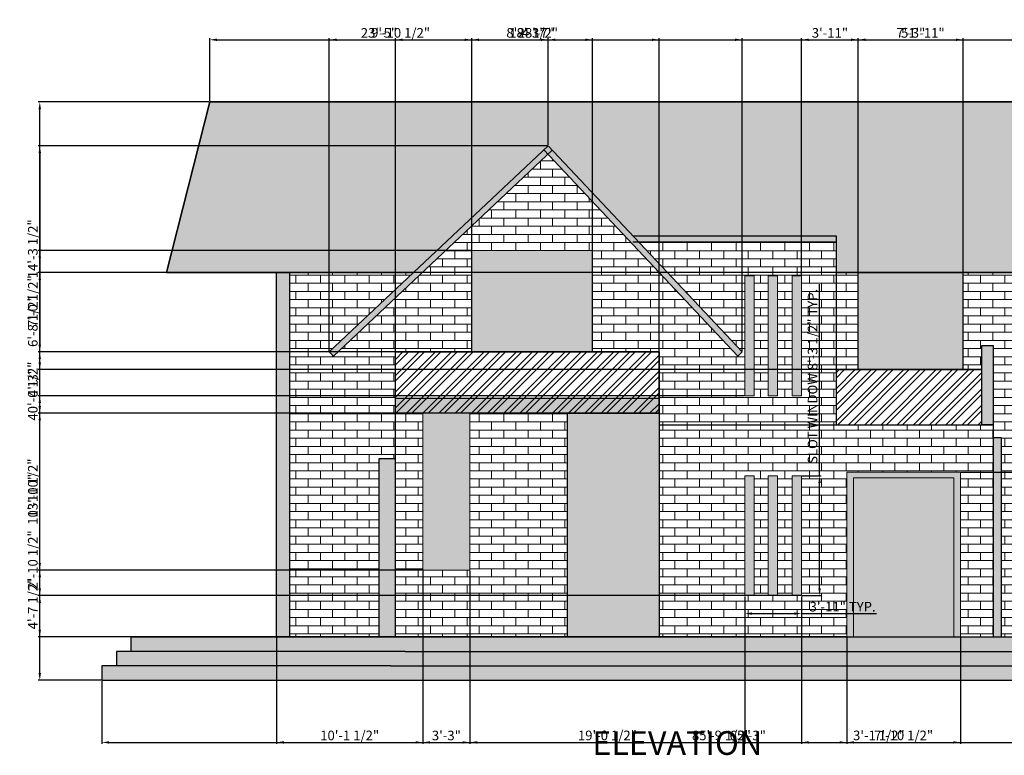
# Model space of a CAD drawing. Units: millimetres. Extents: x 1518 to 2850, y 936 to 2174.
# Tile 1 of 5: x 1518 to 2336, y 936 to 1547. Entities that reach past the tile are written whole.
import ezdxf

# ---------------------------------------------------------------- set-up
doc = ezdxf.new("R2010")
doc.units = ezdxf.units.MM
for name, color, linetype, lineweight, true_color in [('A-ANNO-DIMS', 9, 'Continuous', 18, 0xafd9aa), ('A-ANNO-TEXT', 85, 'Continuous', 25, 0x58ba48), ('A-DOOR', 244, 'Continuous', 20, 0x991b1e), ('A-ELEV-BALC-PATT', 40, 'Continuous', 13, 0xf8d731), ('A-ELEV-BASE-PATT', 251, 'Continuous', 13, 0x636466), ('A-ELEV-PATT', 251, 'Continuous', 13, 0x636466), ('A-ELEV-WALL-PATT', 244, 'Continuous', 13, 0x991b1e), ('A-GLAZ', 141, 'Continuous', 18, 0xadddf7), ('A-ROOF-PATT', 254, 'Continuous', 13, 0xfeeab9)]:
    doc.layers.add(name, color=color, linetype=linetype, lineweight=lineweight, true_color=true_color)
for name, color, linetype, lineweight in [('A-ELEV', 7, 'Continuous', 25), ('A-ELEV-BASE', 7, 'Continuous', 30), ('A-GLAZ-PATT', 141, 'Continuous', 13), ('A-ROOF', 7, 'Continuous', 35)]:
    doc.layers.add(name, color=color, linetype=linetype, lineweight=lineweight)
doc.styles.get("Standard").update_dxf_attribs({"font": 'arial.ttf'})
doc.dimstyles.new('ISO-25', dxfattribs={"dimtxt": 8, "dimasz": 6, "dimexe": 1.25, "dimexo": 0.625, "dimtad": 1, "dimdec": 0, "dimlunit": 3, "dimtxsty": 'Standard', "dimcen": 2.5, "dimadec": 0, "dimazin": 0, "dimtfac": 1, "dimtdec": 0, "dimtmove": 0, "dimatfit": 3, "dimfxl": 1, "dimarcsym": 0})

# ---------------------------------------------------------------- blocks, each defined once
blk = doc.blocks.new('WIN-TRIPLE-SLOT-ELEV')
for points in [[(0, 99.63), (7.73, 99.63), (7.73, 0), (0, 0)], [(19.33, 99.63), (27.06, 99.63), (27.06, 0), (19.33, 0)], [(39.43, 99.63), (47.16, 99.63), (47.16, 0), (39.43, 0)]]:
    blk.add_lwpolyline(points, close=True)
blk = doc.blocks.new('*D30')
at = {"layer": 'A-ANNO-DIMS', "color": 0, "lineweight": -2, "transparency": 16777216}
for p, q in [((2182.71, 1167.89), (2182.71, 1326.95)), ((2168.39, 1167.89), (2183.96, 1167.89)), ((2182.71, 1074.26), (2182.71, 1161.89)), ((2168.39, 1068.26), (2183.96, 1068.26))]:
    blk.add_line(p, q, dxfattribs=at)
at = {"layer": 'A-ANNO-DIMS', "color": 0, "transparency": 16777216}
for points in [[(2181.71, 1161.89), (2183.71, 1161.89), (2182.71, 1167.89)], [(2181.71, 1074.26), (2183.71, 1074.26), (2182.71, 1068.26)]]:
    blk.add_solid(points, dxfattribs=at)
at = {"layer": 'Defpoints', "color": 0, "transparency": 16777216}
for p in [(2167.76, 1167.89), (2182.71, 1167.89), (2167.76, 1068.26)]:
    blk.add_point(p, dxfattribs=at)
at = {"layer": 'A-ANNO-DIMS', "color": 0, "transparency": 16777216, "insert": (2177.94, 1250.42), "char_height": 8, "attachment_point": 5, "rotation": 90}
blk.add_mtext('SLOT WINDOW 8\'-3 1/2" TYP.', dxfattribs=at)
blk = doc.blocks.new('*D31')
at = {"layer": 'A-ANNO-DIMS', "color": 0, "lineweight": -2, "transparency": 16777216}
for p, q in [((2120.6, 1067.64), (2120.6, 1052.07)), ((2167.76, 1067.64), (2167.76, 1052.07)), ((2126.6, 1053.32), (2161.76, 1053.32)), ((2167.76, 1053.32), (2229.98, 1053.32))]:
    blk.add_line(p, q, dxfattribs=at)
at = {"layer": 'A-ANNO-DIMS', "color": 0, "transparency": 16777216}
for points in [[(2126.6, 1054.32), (2126.6, 1052.32), (2120.6, 1053.32)], [(2161.76, 1054.32), (2161.76, 1052.32), (2167.76, 1053.32)]]:
    blk.add_solid(points, dxfattribs=at)
at = {"layer": 'Defpoints', "color": 0, "transparency": 16777216}
for p in [(2120.6, 1068.26), (2167.76, 1068.26), (2167.76, 1053.32)]:
    blk.add_point(p, dxfattribs=at)
at = {"layer": 'A-ANNO-DIMS', "color": 0, "transparency": 16777216, "insert": (2201.87, 1058.03), "char_height": 8, "attachment_point": 5}
blk.add_mtext('3\'-11" TYP.', dxfattribs=at)
blk = doc.blocks.new('*D52')
at = {"layer": 'A-ANNO-DIMS', "color": 0, "lineweight": -2, "transparency": 16777216}
for p, q in [((1852.93, 1088.86), (1852.93, 945.05)), ((1731.47, 1033.32), (1731.47, 945.05)), ((1737.47, 946.3), (1846.93, 946.3))]:
    blk.add_line(p, q, dxfattribs=at)
at = {"layer": 'A-ANNO-DIMS', "color": 0, "transparency": 16777216}
for points in [[(1737.47, 947.3), (1737.47, 945.3), (1731.47, 946.3)], [(1846.93, 947.3), (1846.93, 945.3), (1852.93, 946.3)]]:
    blk.add_solid(points, dxfattribs=at)
at = {"layer": 'Defpoints', "color": 0, "transparency": 16777216}
for p in [(1852.93, 1089.48), (1731.47, 1033.95), (1852.93, 946.3)]:
    blk.add_point(p, dxfattribs=at)
at = {"layer": 'A-ANNO-DIMS', "color": 0, "transparency": 16777216, "insert": (1792.2, 951.06), "char_height": 8, "attachment_point": 5}
blk.add_mtext('10\'-1 1/2"', dxfattribs=at)
blk = doc.blocks.new('*D53')
at = {"layer": 'A-ANNO-DIMS', "color": 0, "lineweight": -2, "transparency": 16777216}
for p, q in [((1852.93, 1088.86), (1852.93, 945.05)), ((1892.17, 1088.86), (1892.17, 945.05)), ((1858.93, 946.3), (1886.17, 946.3))]:
    blk.add_line(p, q, dxfattribs=at)
at = {"layer": 'A-ANNO-DIMS', "color": 0, "transparency": 16777216}
for points in [[(1858.93, 947.3), (1858.93, 945.3), (1852.93, 946.3)], [(1886.17, 947.3), (1886.17, 945.3), (1892.17, 946.3)]]:
    blk.add_solid(points, dxfattribs=at)
at = {"layer": 'Defpoints', "color": 0, "transparency": 16777216}
for p in [(1852.93, 1089.48), (1892.17, 1089.48), (1892.17, 946.3)]:
    blk.add_point(p, dxfattribs=at)
at = {"layer": 'A-ANNO-DIMS', "color": 0, "transparency": 16777216, "insert": (1872.55, 951.01), "char_height": 8, "attachment_point": 5}
blk.add_mtext('3\'-3"', dxfattribs=at)
blk = doc.blocks.new('*D54')
at = {"layer": 'A-ANNO-DIMS', "color": 0, "lineweight": -2, "transparency": 16777216}
for p, q in [((1892.17, 1088.86), (1892.17, 945.05)), ((2120.6, 1067.64), (2120.6, 945.05)), ((1898.17, 946.3), (2114.6, 946.3))]:
    blk.add_line(p, q, dxfattribs=at)
at = {"layer": 'A-ANNO-DIMS', "color": 0, "transparency": 16777216}
for points in [[(1898.17, 947.3), (1898.17, 945.3), (1892.17, 946.3)], [(2114.6, 947.3), (2114.6, 945.3), (2120.6, 946.3)]]:
    blk.add_solid(points, dxfattribs=at)
at = {"layer": 'Defpoints', "color": 0, "transparency": 16777216}
for p in [(1892.17, 1089.48), (2120.6, 1068.26), (2120.6, 946.3)]:
    blk.add_point(p, dxfattribs=at)
at = {"layer": 'A-ANNO-DIMS', "color": 0, "transparency": 16777216, "insert": (2006.39, 951.06), "char_height": 8, "attachment_point": 5}
blk.add_mtext('19\'-0 1/2"', dxfattribs=at)
blk = doc.blocks.new('*D55')
at = {"layer": 'A-ANNO-DIMS', "color": 0, "lineweight": -2, "transparency": 16777216}
for p, q in [((2167.76, 1067.64), (2167.76, 945.05)), ((2205.44, 1033.32), (2205.44, 945.05)), ((2173.76, 946.3), (2199.44, 946.3)), ((2205.44, 946.3), (2252.59, 946.3))]:
    blk.add_line(p, q, dxfattribs=at)
at = {"layer": 'A-ANNO-DIMS', "color": 0, "transparency": 16777216}
for points in [[(2173.76, 947.3), (2173.76, 945.3), (2167.76, 946.3)], [(2199.44, 947.3), (2199.44, 945.3), (2205.44, 946.3)]]:
    blk.add_solid(points, dxfattribs=at)
at = {"layer": 'Defpoints', "color": 0, "transparency": 16777216}
for p in [(2167.76, 1068.26), (2205.44, 1033.95), (2205.44, 946.3)]:
    blk.add_point(p, dxfattribs=at)
at = {"layer": 'A-ANNO-DIMS', "color": 0, "transparency": 16777216, "insert": (2232.01, 951.06), "char_height": 8, "attachment_point": 5}
blk.add_mtext('3\'-1 1/2"', dxfattribs=at)
blk = doc.blocks.new('*D56')
at = {"layer": 'A-ANNO-DIMS', "color": 0, "lineweight": -2, "transparency": 16777216}
for p, q in [((2205.44, 1033.32), (2205.44, 945.05)), ((2299.77, 1033.32), (2299.77, 945.05)), ((2211.44, 946.3), (2293.77, 946.3))]:
    blk.add_line(p, q, dxfattribs=at)
at = {"layer": 'A-ANNO-DIMS', "color": 0, "transparency": 16777216}
for points in [[(2211.44, 947.3), (2211.44, 945.3), (2205.44, 946.3)], [(2293.77, 947.3), (2293.77, 945.3), (2299.77, 946.3)]]:
    blk.add_solid(points, dxfattribs=at)
at = {"layer": 'Defpoints', "color": 0, "transparency": 16777216}
for p in [(2205.44, 1033.95), (2299.77, 1033.95), (2299.77, 946.3)]:
    blk.add_point(p, dxfattribs=at)
at = {"layer": 'A-ANNO-DIMS', "color": 0, "transparency": 16777216, "insert": (2252.6, 951.06), "char_height": 8, "attachment_point": 5}
blk.add_mtext('7\'-10 1/2"', dxfattribs=at)
blk = doc.blocks.new('*D57')
at = {"layer": 'A-ANNO-DIMS', "color": 0, "lineweight": -2, "transparency": 16777216}
for p, q in [((1731.47, 1033.32), (1731.47, 945.05)), ((2514.61, 1033.32), (2514.61, 945.05)), ((1737.47, 946.3), (2508.61, 946.3))]:
    blk.add_line(p, q, dxfattribs=at)
at = {"layer": 'A-ANNO-DIMS', "color": 0, "transparency": 16777216}
for points in [[(1737.47, 947.3), (1737.47, 945.3), (1731.47, 946.3)], [(2508.61, 947.3), (2508.61, 945.3), (2514.61, 946.3)]]:
    blk.add_solid(points, dxfattribs=at)
at = {"layer": 'Defpoints', "color": 0, "transparency": 16777216}
for p in [(1731.47, 1033.95), (2514.61, 1033.95), (2514.61, 946.3)]:
    blk.add_point(p, dxfattribs=at)
at = {"layer": 'A-ANNO-DIMS', "color": 0, "transparency": 16777216, "insert": (2123.04, 951.01), "char_height": 8, "attachment_point": 5}
blk.add_mtext('65\'-3"', dxfattribs=at)
blk = doc.blocks.new('*D58')
at = {"layer": 'A-ANNO-DIMS', "color": 0, "lineweight": -2, "transparency": 16777216}
for p, q in [((2119.98, 1234.32), (1533.38, 1234.32)), ((1534.63, 1074.26), (1534.63, 1228.32)), ((2119.98, 1068.26), (1533.38, 1068.26))]:
    blk.add_line(p, q, dxfattribs=at)
at = {"layer": 'A-ANNO-DIMS', "color": 0, "transparency": 16777216}
for points in [[(1533.63, 1228.32), (1535.63, 1228.32), (1534.63, 1234.32)], [(1533.63, 1074.26), (1535.63, 1074.26), (1534.63, 1068.26)]]:
    blk.add_solid(points, dxfattribs=at)
at = {"layer": 'Defpoints', "color": 0, "transparency": 16777216}
for p in [(1534.63, 1234.32), (2120.6, 1234.32), (2120.6, 1068.26)]:
    blk.add_point(p, dxfattribs=at)
at = {"layer": 'A-ANNO-DIMS', "color": 0, "transparency": 16777216, "insert": (1529.92, 1151.29), "char_height": 8, "attachment_point": 5, "rotation": 90}
blk.add_mtext('13\'-10"', dxfattribs=at)
blk = doc.blocks.new('*D59')
at = {"layer": 'A-ANNO-DIMS', "color": 0, "lineweight": -2, "transparency": 16777216}
for p, q in [((1534.63, 1068.26), (1534.63, 1121.77)), ((2167.14, 1068.26), (1533.38, 1068.26)), ((1534.63, 1039.95), (1534.63, 1062.26)), ((2204.81, 1033.95), (1533.38, 1033.95))]:
    blk.add_line(p, q, dxfattribs=at)
at = {"layer": 'A-ANNO-DIMS', "color": 0, "transparency": 16777216}
for points in [[(1533.63, 1062.26), (1535.63, 1062.26), (1534.63, 1068.26)], [(1533.63, 1039.95), (1535.63, 1039.95), (1534.63, 1033.95)]]:
    blk.add_solid(points, dxfattribs=at)
at = {"layer": 'Defpoints', "color": 0, "transparency": 16777216}
for p in [(1534.63, 1068.26), (2167.76, 1068.26), (2205.44, 1033.95)]:
    blk.add_point(p, dxfattribs=at)
at = {"layer": 'A-ANNO-DIMS', "color": 0, "transparency": 16777216, "insert": (1529.87, 1098.01), "char_height": 8, "attachment_point": 5, "rotation": 90}
blk.add_mtext('2\'-10 1/2"', dxfattribs=at)
blk = doc.blocks.new('*D60')
at = {"layer": 'A-ANNO-DIMS', "color": 0, "lineweight": -2, "transparency": 16777216}
for p, q in [((1852.31, 1219.79), (1533.38, 1219.79)), ((1534.63, 1095.48), (1534.63, 1213.79)), ((1852.31, 1089.48), (1533.38, 1089.48))]:
    blk.add_line(p, q, dxfattribs=at)
at = {"layer": 'A-ANNO-DIMS', "color": 0, "transparency": 16777216}
for points in [[(1533.63, 1213.79), (1535.63, 1213.79), (1534.63, 1219.79)], [(1533.63, 1095.48), (1535.63, 1095.48), (1534.63, 1089.48)]]:
    blk.add_solid(points, dxfattribs=at)
at = {"layer": 'Defpoints', "color": 0, "transparency": 16777216}
for p in [(1534.63, 1219.79), (1852.93, 1219.79), (1852.93, 1089.48)]:
    blk.add_point(p, dxfattribs=at)
at = {"layer": 'A-ANNO-DIMS', "color": 0, "transparency": 16777216, "insert": (1529.87, 1154.64), "char_height": 8, "attachment_point": 5, "rotation": 90}
blk.add_mtext('10\'-10 1/2"', dxfattribs=at)
blk = doc.blocks.new('*D61')
at = {"layer": 'A-ANNO-DIMS', "color": 0, "lineweight": -2, "transparency": 16777216}
for p, q in [((1852.31, 1089.48), (1533.38, 1089.48)), ((1534.63, 1039.95), (1534.63, 1083.48)), ((1730.84, 1033.95), (1533.38, 1033.95))]:
    blk.add_line(p, q, dxfattribs=at)
at = {"layer": 'A-ANNO-DIMS', "color": 0, "transparency": 16777216}
for points in [[(1533.63, 1083.48), (1535.63, 1083.48), (1534.63, 1089.48)], [(1533.63, 1039.95), (1535.63, 1039.95), (1534.63, 1033.95)]]:
    blk.add_solid(points, dxfattribs=at)
at = {"layer": 'Defpoints', "color": 0, "transparency": 16777216}
for p in [(1534.63, 1089.48), (1852.93, 1089.48), (1731.47, 1033.95)]:
    blk.add_point(p, dxfattribs=at)
at = {"layer": 'A-ANNO-DIMS', "color": 0, "transparency": 16777216, "insert": (1529.87, 1061.71), "char_height": 8, "attachment_point": 5, "rotation": 90}
blk.add_mtext('4\'-7 1/2"', dxfattribs=at)
blk = doc.blocks.new('*D62')
at = {"layer": 'A-ANNO-DIMS', "color": 0, "lineweight": -2, "transparency": 16777216}
for p, q in [((1829.69, 1270.74), (1533.38, 1270.74)), ((1534.63, 1225.79), (1534.63, 1264.74)), ((1829.69, 1219.79), (1533.38, 1219.79))]:
    blk.add_line(p, q, dxfattribs=at)
at = {"layer": 'A-ANNO-DIMS', "color": 0, "transparency": 16777216}
for points in [[(1533.63, 1264.74), (1535.63, 1264.74), (1534.63, 1270.74)], [(1533.63, 1225.79), (1535.63, 1225.79), (1534.63, 1219.79)]]:
    blk.add_solid(points, dxfattribs=at)
at = {"layer": 'Defpoints', "color": 0, "transparency": 16777216}
for p in [(1534.63, 1270.74), (1830.31, 1270.74), (1830.31, 1219.79)]:
    blk.add_point(p, dxfattribs=at)
at = {"layer": 'A-ANNO-DIMS', "color": 0, "transparency": 16777216, "insert": (1529.92, 1245.26), "char_height": 8, "attachment_point": 5, "rotation": 90}
blk.add_mtext('4\'-3"', dxfattribs=at)
blk = doc.blocks.new('*D63')
at = {"layer": 'A-ANNO-DIMS', "color": 0, "lineweight": -2, "transparency": 16777216}
for p, q in [((1830.31, 1220.42), (1830.31, 1531.29)), ((2049.41, 1220.42), (2049.41, 1531.29)), ((1836.31, 1530.04), (2043.41, 1530.04))]:
    blk.add_line(p, q, dxfattribs=at)
at = {"layer": 'A-ANNO-DIMS', "color": 0, "transparency": 16777216}
for points in [[(1836.31, 1531.04), (1836.31, 1529.04), (1830.31, 1530.04)], [(2043.41, 1531.04), (2043.41, 1529.04), (2049.41, 1530.04)]]:
    blk.add_solid(points, dxfattribs=at)
at = {"layer": 'Defpoints', "color": 0, "transparency": 16777216}
for p in [(2049.41, 1530.04), (1830.31, 1219.79), (2049.41, 1219.79)]:
    blk.add_point(p, dxfattribs=at)
at = {"layer": 'A-ANNO-DIMS', "color": 0, "transparency": 16777216, "insert": (1939.86, 1534.75), "char_height": 8, "attachment_point": 5}
blk.add_mtext('18\'-3"', dxfattribs=at)
blk = doc.blocks.new('*D64')
at = {"layer": 'A-ANNO-DIMS', "color": 0, "lineweight": -2, "transparency": 16777216}
for p, q in [((2300.4, 1170.72), (2668.93, 1170.72)), ((2667.68, 1039.95), (2667.68, 1164.72)), ((2300.4, 1033.95), (2668.93, 1033.95))]:
    blk.add_line(p, q, dxfattribs=at)
at = {"layer": 'A-ANNO-DIMS', "color": 0, "transparency": 16777216}
for points in [[(2666.68, 1164.72), (2668.68, 1164.72), (2667.68, 1170.72)], [(2666.68, 1039.95), (2668.68, 1039.95), (2667.68, 1033.95)]]:
    blk.add_solid(points, dxfattribs=at)
at = {"layer": 'Defpoints', "color": 0, "transparency": 16777216}
for p in [(2299.77, 1170.72), (2667.68, 1170.72), (2299.77, 1033.95)]:
    blk.add_point(p, dxfattribs=at)
at = {"layer": 'A-ANNO-DIMS', "color": 0, "transparency": 16777216, "insert": (2662.97, 1102.33), "char_height": 8, "attachment_point": 5, "rotation": 90}
blk.add_mtext('11\'-5"', dxfattribs=at)
blk = doc.blocks.new('*D65')
at = {"layer": 'A-ANNO-DIMS', "color": 0, "lineweight": -2, "transparency": 16777216}
for p, q in [((2214.92, 1256.65), (2214.92, 1531.29)), ((2302.13, 1256.65), (2302.13, 1531.29)), ((2220.92, 1530.04), (2296.13, 1530.04))]:
    blk.add_line(p, q, dxfattribs=at)
at = {"layer": 'A-ANNO-DIMS', "color": 0, "transparency": 16777216}
for points in [[(2220.92, 1531.04), (2220.92, 1529.04), (2214.92, 1530.04)], [(2296.13, 1531.04), (2296.13, 1529.04), (2302.13, 1530.04)]]:
    blk.add_solid(points, dxfattribs=at)
at = {"layer": 'Defpoints', "color": 0, "transparency": 16777216}
for p in [(2302.13, 1530.04), (2214.92, 1256.02), (2302.13, 1256.02)]:
    blk.add_point(p, dxfattribs=at)
at = {"layer": 'A-ANNO-DIMS', "color": 0, "transparency": 16777216, "insert": (2258.52, 1534.75), "char_height": 8, "attachment_point": 5}
blk.add_mtext('7\'-3"', dxfattribs=at)
blk = doc.blocks.new('*D66')
at = {"layer": 'A-ANNO-DIMS', "color": 0, "lineweight": -2, "transparency": 16777216}
for p, q in [((2214.29, 1336.6), (1533.38, 1336.6)), ((1534.63, 1262.02), (1534.63, 1330.6)), ((2214.29, 1256.02), (1533.38, 1256.02))]:
    blk.add_line(p, q, dxfattribs=at)
at = {"layer": 'A-ANNO-DIMS', "color": 0, "transparency": 16777216}
for points in [[(1533.63, 1330.6), (1535.63, 1330.6), (1534.63, 1336.6)], [(1533.63, 1262.02), (1535.63, 1262.02), (1534.63, 1256.02)]]:
    blk.add_solid(points, dxfattribs=at)
at = {"layer": 'Defpoints', "color": 0, "transparency": 16777216}
for p in [(1534.63, 1336.6), (2214.92, 1336.6), (2214.92, 1256.02)]:
    blk.add_point(p, dxfattribs=at)
at = {"layer": 'A-ANNO-DIMS', "color": 0, "transparency": 16777216, "insert": (1529.87, 1296.31), "char_height": 8, "attachment_point": 5, "rotation": 90}
blk.add_mtext('6\'-8 1/2"', dxfattribs=at)
blk = doc.blocks.new('*D67')
at = {"layer": 'A-ANNO-DIMS', "color": 0, "lineweight": -2, "transparency": 16777216}
for p, q in [((2167.76, 1334.57), (2167.76, 1531.29)), ((2214.92, 1337.23), (2214.92, 1531.29)), ((2173.76, 1530.04), (2208.92, 1530.04))]:
    blk.add_line(p, q, dxfattribs=at)
at = {"layer": 'A-ANNO-DIMS', "color": 0, "transparency": 16777216}
for points in [[(2173.76, 1531.04), (2173.76, 1529.04), (2167.76, 1530.04)], [(2208.92, 1531.04), (2208.92, 1529.04), (2214.92, 1530.04)]]:
    blk.add_solid(points, dxfattribs=at)
at = {"layer": 'Defpoints', "color": 0, "transparency": 16777216}
for p in [(2214.92, 1530.04), (2167.76, 1333.95), (2214.92, 1336.6)]:
    blk.add_point(p, dxfattribs=at)
at = {"layer": 'A-ANNO-DIMS', "color": 0, "transparency": 16777216, "insert": (2191.34, 1534.75), "char_height": 8, "attachment_point": 5}
blk.add_mtext('3\'-11"', dxfattribs=at)
blk = doc.blocks.new('*D68')
at = {"layer": 'A-ANNO-DIMS', "color": 0, "lineweight": -2, "transparency": 16777216}
for p, q in [((1893.72, 1271.36), (1893.72, 1531.29)), ((1994.04, 1271.36), (1994.04, 1531.29)), ((1899.72, 1530.04), (1988.04, 1530.04))]:
    blk.add_line(p, q, dxfattribs=at)
at = {"layer": 'A-ANNO-DIMS', "color": 0, "transparency": 16777216}
for points in [[(1899.72, 1531.04), (1899.72, 1529.04), (1893.72, 1530.04)], [(1988.04, 1531.04), (1988.04, 1529.04), (1994.04, 1530.04)]]:
    blk.add_solid(points, dxfattribs=at)
at = {"layer": 'Defpoints', "color": 0, "transparency": 16777216}
for p in [(1994.04, 1530.04), (1893.72, 1270.74), (1994.04, 1270.74)]:
    blk.add_point(p, dxfattribs=at)
at = {"layer": 'A-ANNO-DIMS', "color": 0, "transparency": 16777216, "insert": (1943.88, 1534.8), "char_height": 8, "attachment_point": 5}
blk.add_mtext('8\'-4 1/2"', dxfattribs=at)
blk = doc.blocks.new('*D69')
at = {"layer": 'A-ANNO-DIMS', "color": 0, "lineweight": -2, "transparency": 16777216}
for p, q in [((1893.1, 1355.03), (1533.38, 1355.03)), ((1534.63, 1276.74), (1534.63, 1349.03)), ((1893.1, 1270.74), (1533.38, 1270.74))]:
    blk.add_line(p, q, dxfattribs=at)
at = {"layer": 'A-ANNO-DIMS', "color": 0, "transparency": 16777216}
for points in [[(1533.63, 1349.03), (1535.63, 1349.03), (1534.63, 1355.03)], [(1533.63, 1276.74), (1535.63, 1276.74), (1534.63, 1270.74)]]:
    blk.add_solid(points, dxfattribs=at)
at = {"layer": 'Defpoints', "color": 0, "transparency": 16777216}
for p in [(1534.63, 1355.03), (1893.72, 1355.03), (1893.72, 1270.74)]:
    blk.add_point(p, dxfattribs=at)
at = {"layer": 'A-ANNO-DIMS', "color": 0, "transparency": 16777216, "insert": (1529.87, 1312.88), "char_height": 8, "attachment_point": 5, "rotation": 90}
blk.add_mtext('7\'-0 1/2"', dxfattribs=at)
blk = doc.blocks.new('*D70')
at = {"layer": 'A-ANNO-DIMS', "color": 0, "lineweight": -2, "transparency": 16777216}
for p, q in [((1775.28, 1271.36), (1775.28, 1531.29)), ((1893.72, 1271.36), (1893.72, 1531.29)), ((1781.28, 1530.04), (1887.72, 1530.04))]:
    blk.add_line(p, q, dxfattribs=at)
at = {"layer": 'A-ANNO-DIMS', "color": 0, "transparency": 16777216}
for points in [[(1781.28, 1531.04), (1781.28, 1529.04), (1775.28, 1530.04)], [(1887.72, 1531.04), (1887.72, 1529.04), (1893.72, 1530.04)]]:
    blk.add_solid(points, dxfattribs=at)
at = {"layer": 'Defpoints', "color": 0, "transparency": 16777216}
for p in [(1893.72, 1530.04), (1775.28, 1270.74), (1893.72, 1270.74)]:
    blk.add_point(p, dxfattribs=at)
at = {"layer": 'A-ANNO-DIMS', "color": 0, "transparency": 16777216, "insert": (1834.5, 1534.8), "char_height": 8, "attachment_point": 5}
blk.add_mtext('9\'-10 1/2"', dxfattribs=at)
blk = doc.blocks.new('*D71')
at = {"layer": 'A-ANNO-DIMS', "color": 0, "lineweight": -2, "transparency": 16777216}
for p, q in [((1775.28, 1271.36), (1775.28, 1531.29)), ((2118.49, 1271.36), (2118.49, 1531.29)), ((1781.28, 1530.04), (2112.49, 1530.04))]:
    blk.add_line(p, q, dxfattribs=at)
at = {"layer": 'A-ANNO-DIMS', "color": 0, "transparency": 16777216}
for points in [[(1781.28, 1531.04), (1781.28, 1529.04), (1775.28, 1530.04)], [(2112.49, 1531.04), (2112.49, 1529.04), (2118.49, 1530.04)]]:
    blk.add_solid(points, dxfattribs=at)
at = {"layer": 'Defpoints', "color": 0, "transparency": 16777216}
for p in [(2118.49, 1530.04), (1775.28, 1270.74), (2118.49, 1270.74)]:
    blk.add_point(p, dxfattribs=at)
at = {"layer": 'A-ANNO-DIMS', "color": 0, "transparency": 16777216, "insert": (1946.88, 1534.75), "char_height": 8, "attachment_point": 5}
blk.add_mtext('28\'-7"', dxfattribs=at)
blk = doc.blocks.new('*D72')
at = {"layer": 'A-ANNO-DIMS', "color": 0, "lineweight": -2, "transparency": 16777216}
for p, q in [((1956.5, 1442.04), (1533.38, 1442.04)), ((1534.63, 1436.04), (1534.63, 1276.74)), ((1774.65, 1270.74), (1533.38, 1270.74))]:
    blk.add_line(p, q, dxfattribs=at)
at = {"layer": 'A-ANNO-DIMS', "color": 0, "transparency": 16777216}
for points in [[(1533.63, 1436.04), (1535.63, 1436.04), (1534.63, 1442.04)], [(1533.63, 1276.74), (1535.63, 1276.74), (1534.63, 1270.74)]]:
    blk.add_solid(points, dxfattribs=at)
at = {"layer": 'Defpoints', "color": 0, "transparency": 16777216}
for p in [(1957.13, 1442.04), (1534.63, 1270.74), (1775.28, 1270.74)]:
    blk.add_point(p, dxfattribs=at)
at = {"layer": 'A-ANNO-DIMS', "color": 0, "transparency": 16777216, "insert": (1529.86, 1356.39), "char_height": 8, "attachment_point": 5, "rotation": 90}
blk.add_mtext('14\'-3 1/2"', dxfattribs=at)
blk = doc.blocks.new('*D73')
at = {"layer": 'A-ANNO-DIMS', "color": 0, "lineweight": -2, "transparency": 16777216}
for p, q in [((1675.89, 1479.02), (1675.89, 1531.29)), ((1957.13, 1442.66), (1957.13, 1531.29)), ((1681.89, 1530.04), (1951.13, 1530.04))]:
    blk.add_line(p, q, dxfattribs=at)
at = {"layer": 'A-ANNO-DIMS', "color": 0, "transparency": 16777216}
for points in [[(1681.89, 1531.04), (1681.89, 1529.04), (1675.89, 1530.04)], [(1951.13, 1531.04), (1951.13, 1529.04), (1957.13, 1530.04)]]:
    blk.add_solid(points, dxfattribs=at)
at = {"layer": 'Defpoints', "color": 0, "transparency": 16777216}
for p in [(1957.13, 1530.04), (1675.89, 1478.39), (1957.13, 1442.04)]:
    blk.add_point(p, dxfattribs=at)
at = {"layer": 'A-ANNO-DIMS', "color": 0, "transparency": 16777216, "insert": (1816.51, 1534.75), "char_height": 8, "attachment_point": 5}
blk.add_mtext('23\'-5"', dxfattribs=at)
blk = doc.blocks.new('*D74')
at = {"layer": 'A-ANNO-DIMS', "color": 0, "lineweight": -2, "transparency": 16777216}
for p, q in [((1957.13, 1442.66), (1957.13, 1531.29)), ((2580.03, 1479.02), (2580.03, 1531.29)), ((1963.13, 1530.04), (2574.03, 1530.04))]:
    blk.add_line(p, q, dxfattribs=at)
at = {"layer": 'A-ANNO-DIMS', "color": 0, "transparency": 16777216}
for points in [[(1963.13, 1531.04), (1963.13, 1529.04), (1957.13, 1530.04)], [(2574.03, 1531.04), (2574.03, 1529.04), (2580.03, 1530.04)]]:
    blk.add_solid(points, dxfattribs=at)
at = {"layer": 'Defpoints', "color": 0, "transparency": 16777216}
for p in [(2580.03, 1530.04), (2580.03, 1478.39), (1957.13, 1442.04)]:
    blk.add_point(p, dxfattribs=at)
at = {"layer": 'A-ANNO-DIMS', "color": 0, "transparency": 16777216, "insert": (2268.58, 1534.75), "char_height": 8, "attachment_point": 5}
blk.add_mtext('51\'-11"', dxfattribs=at)
blk = doc.blocks.new('*D77')
at = {"layer": 'A-ANNO-DIMS', "color": 0, "lineweight": -2, "transparency": 16777216}
for p, q in [((2616.03, 1335.98), (2616.03, 945.05)), ((1586.28, 997.32), (1586.28, 945.05)), ((1592.28, 946.3), (2610.03, 946.3))]:
    blk.add_line(p, q, dxfattribs=at)
at = {"layer": 'A-ANNO-DIMS', "color": 0, "transparency": 16777216}
for points in [[(1592.28, 947.3), (1592.28, 945.3), (1586.28, 946.3)], [(2610.03, 947.3), (2610.03, 945.3), (2616.03, 946.3)]]:
    blk.add_solid(points, dxfattribs=at)
at = {"layer": 'Defpoints', "color": 0, "transparency": 16777216}
for p in [(2616.03, 1336.6), (1586.28, 997.95), (2616.03, 946.3)]:
    blk.add_point(p, dxfattribs=at)
at = {"layer": 'A-ANNO-DIMS', "color": 0, "transparency": 16777216, "insert": (2101.15, 951.06), "char_height": 8, "attachment_point": 5}
blk.add_mtext('85\'-9 1/2"', dxfattribs=at)
blk = doc.blocks.new('*D78')
at = {"layer": 'A-ANNO-DIMS', "color": 0, "lineweight": -2, "transparency": 16777216}
for p, q in [((1675.27, 1478.39), (1533.38, 1478.39)), ((1534.63, 1003.95), (1534.63, 1472.39)), ((1585.65, 997.95), (1533.38, 997.95))]:
    blk.add_line(p, q, dxfattribs=at)
at = {"layer": 'A-ANNO-DIMS', "color": 0, "transparency": 16777216}
for points in [[(1533.63, 1472.39), (1535.63, 1472.39), (1534.63, 1478.39)], [(1533.63, 1003.95), (1535.63, 1003.95), (1534.63, 997.95)]]:
    blk.add_solid(points, dxfattribs=at)
at = {"layer": 'Defpoints', "color": 0, "transparency": 16777216}
for p in [(1534.63, 1478.39), (1675.89, 1478.39), (1586.28, 997.95)]:
    blk.add_point(p, dxfattribs=at)
at = {"layer": 'A-ANNO-DIMS', "color": 0, "transparency": 16777216, "insert": (1529.87, 1238.17), "char_height": 8, "attachment_point": 5, "rotation": 90}
blk.add_mtext('40\'-0 1/2"', dxfattribs=at)

msp = doc.modelspace()

# ---------------------------------------------------------------- hatches: boundary and pattern name
at = {"layer": 'A-ELEV-BALC-PATT'}
h = msp.add_hatch(dxfattribs=at)
h.set_pattern_fill('ANSI32', color=256, style=0)
h.paths.add_polyline_path([(2049.41, 1270.74), (1830.31, 1270.74), (1830.31, 1232.28), (2049.41, 1232.28)])
h.paths.add_polyline_path([(2317.67, 1256.02), (2196.4, 1256.02), (2196.4, 1210.06), (2317.67, 1210.06)])
h.paths.add_polyline_path([(2049.41, 1232.28), (1830.31, 1232.28), (1830.31, 1219.79), (2049.41, 1219.79)])
at = {"layer": 'A-ELEV-BASE-PATT'}
h = msp.add_hatch(dxfattribs=at)
h.set_pattern_fill('AR-SAND', color=256, scale=0.01, style=0)
h.paths.add_polyline_path([(2536.2, 1033.95), (1610.28, 1033.95), (1610.28, 1021.95), (1838.28, 1021.95), (2536.2, 1021.95)])
h.paths.add_polyline_path([(2548.2, 1021.95), (2536.2, 1021.95), (1838.28, 1021.95), (1598.28, 1021.95), (1598.28, 1009.95), (1826.28, 1009.95), (2548.2, 1009.95)])
h.paths.add_polyline_path([(2560.2, 1009.95), (2548.2, 1009.95), (1826.28, 1009.95), (1586.28, 1009.95), (1586.28, 997.95), (2560.2, 997.95)])
at = {"layer": 'A-ELEV-PATT'}
h = msp.add_hatch(dxfattribs=at)
h.set_pattern_fill('ANSI33', color=256, style=0)
h.paths.add_polyline_path([(1830.31, 1182.15), (1816.59, 1182.15), (1816.59, 1033.95), (1830.31, 1033.95)])
h.paths.add_polyline_path([(2049.41, 1219.79), (1973.1, 1219.79), (1973.1, 1033.95), (2049.41, 1033.95)])
h.paths.add_polyline_path([(2299.77, 1170.72), (2205.44, 1170.72), (2205.44, 1033.95), (2210.83, 1033.95), (2210.83, 1166.04), (2294.18, 1166.04), (2294.18, 1033.95), (2299.77, 1033.95)])
h.paths.add_polyline_path([(2334.04, 1199.48), (2326.9, 1199.48), (2326.9, 1033.95), (2334.04, 1033.95)])
h.paths.add_polyline_path([(2326.9, 1275.95), (2317.67, 1275.95), (2317.67, 1210.06), (2326.9, 1210.06)])
h.paths.add_polyline_path([(2196.4, 1367.18), (2027.64, 1367.18), (2032.35, 1362.18), (2196.4, 1362.18)])
h.paths.add_polyline_path([(1960.55, 1438.4), (1956.91, 1434.97), (2114.85, 1267.31), (2118.49, 1270.74)])
h.paths.add_polyline_path([(1956.91, 1434.97), (1953.49, 1438.61), (1775.28, 1270.74), (1778.71, 1267.1)])
h.paths.add_polyline_path([(1957.13, 1442.04), (1953.49, 1438.61), (1956.91, 1434.97), (1960.55, 1438.4)])
h.paths.add_polyline_path([(1742.14, 1336.6), (1731.47, 1336.6), (1731.47, 1033.95), (1742.14, 1033.95)])
h = msp.add_hatch(dxfattribs=at)
h.set_pattern_fill('AR-SAND', color=256, scale=0.01, style=0)
h.paths.add_polyline_path([(1830.31, 1182.15), (1816.59, 1182.15), (1816.59, 1033.95), (1830.31, 1033.95)])
h.paths.add_polyline_path([(1956.91, 1434.97), (1953.49, 1438.61), (1775.28, 1270.74), (1778.71, 1267.1)])
h.paths.add_polyline_path([(1960.55, 1438.4), (1956.91, 1434.97), (2114.85, 1267.31), (2118.49, 1270.74)])
h.paths.add_polyline_path([(2196.4, 1367.18), (2027.64, 1367.18), (2032.35, 1362.18), (2196.4, 1362.18)])
h.paths.add_polyline_path([(2326.9, 1275.95), (2317.67, 1275.95), (2317.67, 1210.06), (2326.9, 1210.06)])
h.paths.add_polyline_path([(2334.04, 1199.48), (2326.9, 1199.48), (2326.9, 1033.95), (2334.04, 1033.95)])
h.paths.add_polyline_path([(2299.77, 1170.72), (2205.44, 1170.72), (2205.44, 1033.95), (2210.83, 1033.95), (2210.83, 1166.04), (2294.18, 1166.04), (2294.18, 1033.95), (2299.77, 1033.95)])
h.paths.add_polyline_path([(2049.41, 1232.28), (1830.31, 1232.28), (1830.31, 1219.79), (2049.41, 1219.79)])
h.paths.add_polyline_path([(1742.14, 1336.6), (1731.47, 1336.6), (1731.47, 1033.95), (1742.14, 1033.95)])
at = {"layer": 'A-ELEV-WALL-PATT'}
h = msp.add_hatch(dxfattribs=at)
h.set_pattern_fill('AR-BRSTD', color=256, scale=0.1)
h.paths.add_polyline_path([(1830.31, 1270.74), (1893.72, 1270.74), (1893.72, 1355.03), (1994.04, 1355.03), (1994.04, 1270.74), (2049.41, 1270.74), (2049.41, 1210.06), (2196.4, 1210.06), (2196.4, 1362.18), (2032.35, 1362.18), (2118.49, 1270.74), (2114.85, 1267.31), (1956.91, 1434.97), (1778.71, 1267.1), (1775.28, 1270.74), (1845.2, 1336.6), (1742.14, 1336.6), (1742.14, 1033.95), (1816.59, 1033.95), (1816.59, 1182.15), (1830.31, 1182.15)])
h.paths.add_polyline_path([(2120.6, 1234.32), (2120.6, 1333.95), (2128.33, 1333.95), (2128.33, 1234.32)], flags=16)
h.paths.add_polyline_path([(2139.93, 1234.32), (2139.93, 1333.95), (2147.66, 1333.95), (2147.66, 1234.32)], flags=16)
h.paths.add_polyline_path([(2160.03, 1234.32), (2160.03, 1333.95), (2167.76, 1333.95), (2167.76, 1234.32)], flags=16)
h.paths.add_polyline_path([(2514.61, 1336.6), (2302.13, 1336.6), (2302.13, 1256.02), (2317.67, 1256.02), (2317.67, 1275.95), (2326.9, 1275.95), (2326.9, 1210.06), (2326.9, 1199.48), (2334.04, 1199.48), (2334.04, 1033.95), (2514.61, 1033.95)])
h.paths.add_polyline_path([(2214.92, 1336.6), (2196.4, 1336.6), (2196.4, 1256.02), (2214.92, 1256.02)])
h.paths.add_polyline_path([(2205.44, 1170.72), (2299.77, 1170.72), (2299.77, 1033.95), (2326.9, 1033.95), (2326.9, 1199.48), (2326.9, 1210.06), (2317.67, 1210.06), (2049.41, 1210.06), (2049.41, 1033.95), (2205.44, 1033.95)])
h.paths.add_polyline_path([(2120.6, 1167.89), (2128.33, 1167.89), (2128.33, 1068.26), (2120.6, 1068.26)], flags=16)
h.paths.add_polyline_path([(2139.93, 1167.89), (2147.66, 1167.89), (2147.66, 1068.26), (2139.93, 1068.26)], flags=16)
h.paths.add_polyline_path([(2160.03, 1167.89), (2167.76, 1167.89), (2167.76, 1068.26), (2160.03, 1068.26)], flags=16)
h.paths.add_polyline_path([(1973.1, 1219.79), (1892.17, 1219.79), (1892.17, 1089.48), (1852.93, 1089.48), (1852.93, 1219.79), (1830.31, 1219.79), (1830.31, 1182.15), (1830.31, 1033.95), (1973.1, 1033.95)], flags=17)
at = {"layer": 'A-GLAZ-PATT'}
h = msp.add_hatch(color=256, dxfattribs=at)
h.set_gradient(color1=(173, 221, 247), color2=(122, 175, 223), name='INVCYLINDER')
h.paths.add_polyline_path([(1994.04, 1270.74), (1994.04, 1355.03), (1893.72, 1355.03), (1893.72, 1270.74)])
h.paths.add_polyline_path([(1852.93, 1089.48), (1892.17, 1089.48), (1892.17, 1219.79), (1852.93, 1219.79)])
h.paths.add_polyline_path([(2214.92, 1256.02), (2302.13, 1256.02), (2302.13, 1336.6), (2214.92, 1336.6)])
h.paths.add_polyline_path([(2210.83, 1033.95), (2294.18, 1033.95), (2294.18, 1166.04), (2210.83, 1166.04)])
h = msp.add_hatch(color=256, dxfattribs=at)
h.set_gradient(color1=(173, 221, 247), color2=(122, 175, 223), name='INVCYLINDER')
h.paths.add_polyline_path([(2120.6, 1234.32), (2128.33, 1234.32), (2128.33, 1333.95), (2120.6, 1333.95)])
h.paths.add_polyline_path([(2147.66, 1333.95), (2139.93, 1333.95), (2139.93, 1234.32), (2147.66, 1234.32)])
h.paths.add_polyline_path([(2160.03, 1234.32), (2167.76, 1234.32), (2167.76, 1333.95), (2160.03, 1333.95)])
h.paths.add_polyline_path([(2128.33, 1167.89), (2120.6, 1167.89), (2120.6, 1068.26), (2128.33, 1068.26)])
h.paths.add_polyline_path([(2147.66, 1167.89), (2139.93, 1167.89), (2139.93, 1068.26), (2147.66, 1068.26)])
h.paths.add_polyline_path([(2160.03, 1068.26), (2167.76, 1068.26), (2167.76, 1167.89), (2160.03, 1167.89)])
at = {"layer": 'A-ROOF-PATT'}
h = msp.add_hatch(dxfattribs=at)
h.set_pattern_fill('AR-RROOF', color=256, scale=0.2)
h.paths.add_polyline_path([(1957.13, 1442.04), (2027.64, 1367.18), (2196.4, 1367.18), (2196.4, 1336.6), (2514.61, 1336.6), (2616.03, 1336.6), (2580.03, 1478.39), (1675.89, 1478.39), (1639.89, 1336.6), (1845.2, 1336.6)])

# ---------------------------------------------------------------- linework, layer by layer
at = {"layer": 'A-DOOR'}
for points in [[(2205.44, 1033.95), (2299.77, 1033.95), (2299.77, 1170.72), (2205.44, 1170.72)], [(2210.83, 1033.95), (2294.18, 1033.95), (2294.18, 1166.04), (2210.83, 1166.04)]]:
    msp.add_lwpolyline(points, close=True, dxfattribs=at)
at = {"layer": 'A-ELEV'}
for p, q in [((2027.64, 1367.18), (2196.4, 1367.18)), ((2196.4, 1367.18), (2196.4, 1210.06)), ((2027.64, 1362.18), (2196.4, 1362.18)), ((1731.47, 1033.95), (1731.47, 1336.6)), ((1742.14, 1336.6), (1742.14, 1033.95)), ((1830.31, 1033.95), (1830.31, 1270.74)), ((2049.41, 1270.74), (2049.41, 1033.95)), ((1830.31, 1232.28), (2049.41, 1232.28)), ((2049.41, 1232.28), (2049.41, 1219.79)), ((2049.41, 1219.79), (1830.31, 1219.79)), ((2049.41, 1210.06), (2326.9, 1210.06)), ((2326.9, 1210.06), (2326.9, 1033.95)), ((1816.59, 1033.95), (1816.59, 1182.15)), ((1816.59, 1182.15), (1830.31, 1182.15)), ((1742.14, 1033.95), (1731.47, 1033.95)), ((1830.31, 1033.95), (1816.59, 1033.95))]:
    msp.add_line(p, q, dxfattribs=at)
for points in [[(1830.31, 1270.74), (2049.41, 1270.74), (2049.41, 1270.74), (1830.31, 1270.74)], [(2326.9, 1210.06), (2317.67, 1210.06), (2317.67, 1275.95), (2326.9, 1275.95)], [(2317.67, 1256.02), (2196.4, 1256.02), (2196.4, 1256.02), (2317.67, 1256.02)], [(1973.1, 1219.79), (2049.41, 1219.79), (2049.41, 1033.95), (1973.1, 1033.95)], [(2326.9, 1210.06), (2326.9, 1210.06), (2326.9, 1210.06), (2326.9, 1210.06)], [(2326.9, 1033.95), (2334.04, 1033.95), (2334.04, 1199.48), (2326.9, 1199.48)]]:
    msp.add_lwpolyline(points, close=True, dxfattribs=at)
at = {"layer": 'A-ELEV-BASE'}
for p, q in [((1610.28, 1033.95), (2536.2, 1033.95)), ((1610.28, 1033.95), (1610.28, 1021.95)), ((1838.28, 1021.95), (1598.28, 1021.95)), ((1598.28, 1021.95), (1598.28, 1009.95)), ((1838.28, 1021.95), (2536.2, 1021.95)), ((1826.28, 1009.95), (1586.28, 1009.95)), ((1586.28, 1009.95), (1586.28, 997.95)), ((1826.28, 1009.95), (2548.2, 1009.95)), ((1586.28, 997.95), (2560.2, 997.95))]:
    msp.add_line(p, q, dxfattribs=at)
at = {"layer": 'A-GLAZ'}
for points in [[(1893.72, 1355.03), (1994.04, 1355.03), (1994.04, 1270.74), (1893.72, 1270.74)], [(2214.92, 1336.6), (2302.13, 1336.6), (2302.13, 1256.02), (2214.92, 1256.02)], [(1852.93, 1219.79), (1892.17, 1219.79), (1892.17, 1089.48), (1852.93, 1089.48)]]:
    msp.add_lwpolyline(points, close=True, dxfattribs=at)
at = {"layer": 'A-ROOF'}
for p, q in [((1675.89, 1478.39), (1639.89, 1336.6)), ((2580.03, 1478.39), (1675.89, 1478.39)), ((1957.13, 1442.04), (1775.28, 1270.74)), ((1957.13, 1442.04), (1957.13, 1442.04)), ((1957.13, 1442.04), (2118.49, 1270.74)), ((1960.55, 1438.4), (1778.71, 1267.1)), ((1953.49, 1438.61), (2114.85, 1267.31)), ((1639.89, 1336.6), (1845.2, 1336.6)), ((2514.61, 1336.6), (2196.4, 1336.6)), ((1775.28, 1270.74), (1778.71, 1267.1)), ((2114.85, 1267.31), (2118.49, 1270.74))]:
    msp.add_line(p, q, dxfattribs=at)

# ---------------------------------------------------------------- block references
at = {"layer": 'A-GLAZ'}
for p in [(2120.6, 1234.32), (2120.6, 1068.26)]:
    msp.add_blockref('WIN-TRIPLE-SLOT-ELEV', p, dxfattribs=at)

# ---------------------------------------------------------------- texts
at = {"layer": 'A-ANNO-TEXT'}
msp.add_text('ELEVATION', height=19.688, dxfattribs=at).set_placement((1993.8, 935.94))

# ---------------------------------------------------------------- dimensions: what is measured, and where the dimension line sits
at = {"layer": 'A-ANNO-DIMS'}
for base, p1, p2, picture, middle in [((1893.72, 1530.04), (1775.28, 1270.74), (1893.72, 1270.74), '*D70', (1834.5, 1534.8)), ((1994.04, 1530.04), (1893.72, 1270.74), (1994.04, 1270.74), '*D68', (1943.88, 1534.8)), ((1957.13, 1530.04), (1675.89, 1478.39), (1957.13, 1442.04), '*D73', (1816.51, 1534.75)), ((2118.49, 1530.04), (1775.28, 1270.74), (2118.49, 1270.74), '*D71', (1946.88, 1534.75)), ((2049.41, 1530.04), (1830.31, 1219.79), (2049.41, 1219.79), '*D63', (1939.86, 1534.75)), ((2580.03, 1530.04), (1957.13, 1442.04), (2580.03, 1478.39), '*D74', (2268.58, 1534.75)), ((2214.92, 1530.04), (2167.76, 1333.95), (2214.92, 1336.6), '*D67', (2191.34, 1534.75)), ((2302.13, 1530.04), (2214.92, 1256.02), (2302.13, 1256.02), '*D65', (2258.52, 1534.75)), ((2616.027, 946.2961), (1586.2782, 997.9461), (2616.027, 1336.6004), '*D77', (2101.1526, 951.0575)), ((1852.93, 946.3), (1731.47, 1033.95), (1852.93, 1089.48), '*D52', (1792.2, 951.06)), ((1892.17, 946.3), (1852.93, 1089.48), (1892.17, 1089.48), '*D53', (1872.55, 951.01)), ((2120.6, 946.3), (1892.17, 1089.48), (2120.6, 1068.26), '*D54', (2006.39, 951.06)), ((2205.44, 946.3), (2167.76, 1068.26), (2205.44, 1033.95), '*D55', (2232.01, 951.06)), ((2514.61, 946.3), (1731.47, 1033.95), (2514.61, 1033.95), '*D57', (2123.04, 951.01)), ((2299.77, 946.3), (2205.44, 1033.95), (2299.77, 1033.95), '*D56', (2252.6, 951.06))]:
    dim = msp.add_linear_dim(base=base, p1=p1, p2=p2, dimstyle='ISO-25', override={"dimdec": 1, "dimlfac": 1, "dimrnd": 0, "dimzin": 1, "dimdsep": 46, "dimlunit": 4, "dimfrac": 2}, dxfattribs=at)
    dim.commit()
    dim.dimension.update_dxf_attribs({"geometry": picture, "text_midpoint": middle})
for base, p1, p2, picture, middle in [((1534.63, 1478.39), (1586.28, 997.95), (1675.89, 1478.39), '*D78', (1529.87, 1238.17)), ((1534.63, 1270.74), (1957.13, 1442.04), (1775.28, 1270.74), '*D72', (1529.86, 1356.39)), ((1534.63, 1355.03), (1893.72, 1270.74), (1893.72, 1355.03), '*D69', (1529.87, 1312.88)), ((1534.63, 1336.6), (2214.92, 1256.02), (2214.92, 1336.6), '*D66', (1529.87, 1296.31)), ((1534.6282, 1270.7358), (1830.3135, 1219.7925), (1830.3135, 1270.7358), '*D62', (1529.9159, 1245.2642)), ((1534.63, 1234.32), (2120.6, 1068.26), (2120.6, 1234.32), '*D58', (1529.92, 1151.29)), ((1534.63, 1219.79), (1852.93, 1089.48), (1852.93, 1219.79), '*D60', (1529.87, 1154.64)), ((2667.68, 1170.72), (2299.77, 1033.95), (2299.77, 1170.72), '*D64', (2662.97, 1102.33)), ((1534.63, 1068.26), (2205.44, 1033.95), (2167.76, 1068.26), '*D59', (1529.87, 1098.01)), ((1534.63, 1089.48), (1731.47, 1033.95), (1852.93, 1089.48), '*D61', (1529.87, 1061.71))]:
    dim = msp.add_linear_dim(base=base, p1=p1, p2=p2, angle=90, dimstyle='ISO-25', override={"dimdec": 1, "dimlfac": 1, "dimrnd": 0, "dimzin": 1, "dimdsep": 46, "dimlunit": 4, "dimfrac": 2}, dxfattribs=at)
    dim.commit()
    dim.dimension.update_dxf_attribs({"geometry": picture, "text_midpoint": middle})
dim = msp.add_linear_dim(base=(2182.71, 1167.89), p1=(2167.76, 1068.26), p2=(2167.76, 1167.89), angle=90, text='SLOT WINDOW <> TYP.', dimstyle='ISO-25', override={"dimdec": 1, "dimlfac": 1, "dimrnd": 0, "dimzin": 1, "dimdsep": 46, "dimlunit": 4, "dimfrac": 2}, dxfattribs=at)
dim.commit()
dim.dimension.update_dxf_attribs({"geometry": '*D30', "text_midpoint": (2177.94, 1250.42)})
dim = msp.add_linear_dim(base=(2167.76, 1053.32), p1=(2120.6, 1068.26), p2=(2167.76, 1068.26), text='<> TYP.', dimstyle='ISO-25', override={"dimdec": 1, "dimlfac": 1, "dimrnd": 0, "dimzin": 1, "dimdsep": 46, "dimlunit": 4, "dimfrac": 2}, dxfattribs=at)
dim.commit()
dim.dimension.update_dxf_attribs({"geometry": '*D31', "text_midpoint": (2201.87, 1058.03)})

doc.saveas('drawing.dxf')
